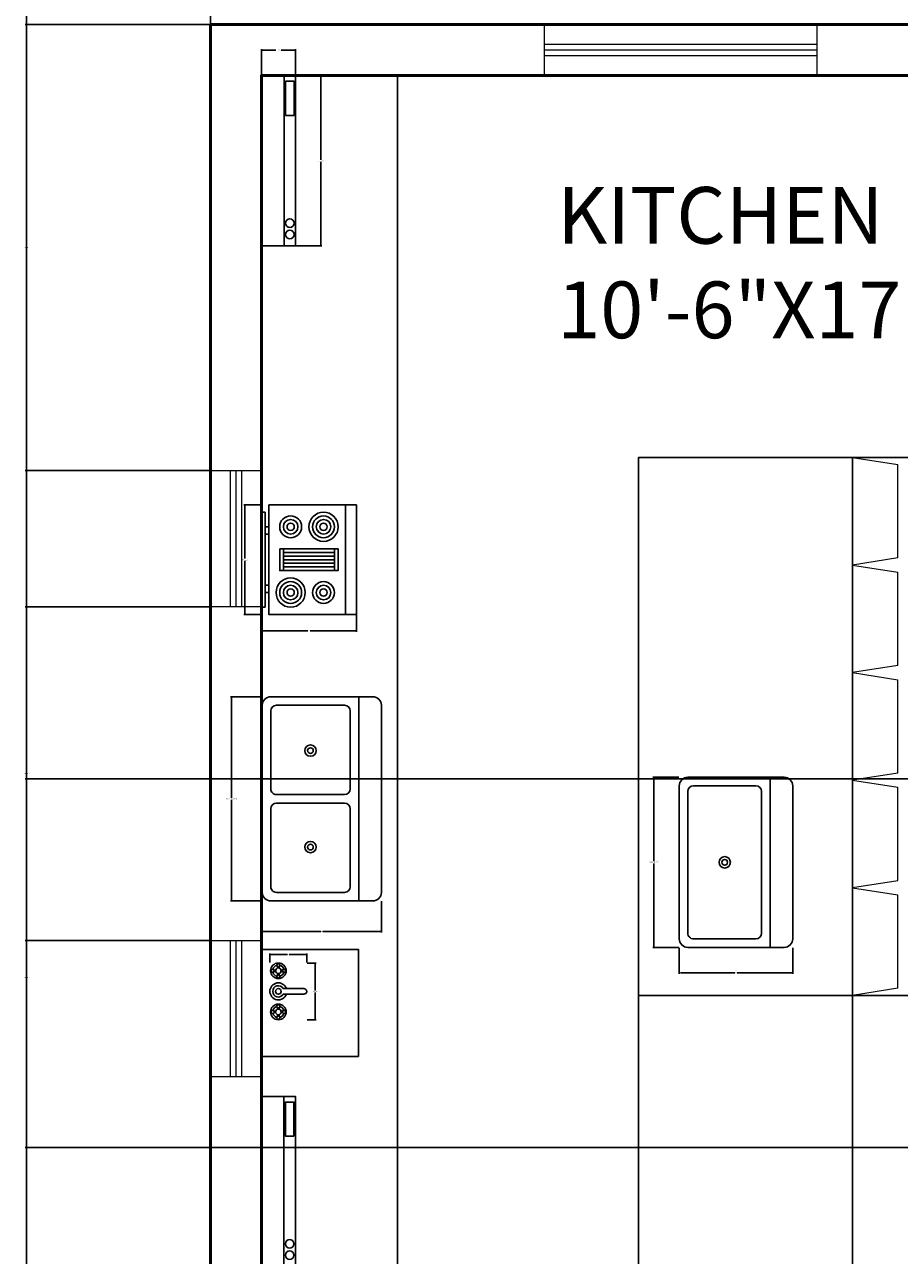
# Model space of a CAD drawing. Units: inches. Extents: x 821 to 2399, y 74 to 823.
# Tile 3 of 13: x 821 to 975, y 381 to 599. Entities that reach past the tile are written whole.
import ezdxf

# ---------------------------------------------------------------- set-up
doc = ezdxf.new("R2010")
doc.units = ezdxf.units.IN
doc.header["$MEASUREMENT"] = 0
doc.layers.get('0').update_dxf_attribs({"lineweight": 53})
for name, color, linetype, lineweight in [('A-ANNO-DIMS', 2, 'Continuous', 18), ('A-AREA-IDEN', 7, 'Continuous', 18), ('A-EQPM', 9, 'Continuous', 25), ('A-FLOR-CASE', 9, 'Continuous', 25), ('A-FLOR-FIXT', 8, 'Continuous', 25), ('A-FURN', 8, 'Continuous', 18), ('A-GLAZ', 4, 'Continuous', 18), ('WALLS', 7, 'Continuous', 50)]:
    doc.layers.add(name, color=color, linetype=linetype, lineweight=lineweight)
doc.styles.get("Standard").update_dxf_attribs({"font": 'arial.ttf'})
doc.dimstyles.get("Standard").update_dxf_attribs({"dimtxt": 0.18, "dimasz": 0.18, "dimexe": 0.18, "dimexo": 0.0625, "dimgap": 0.09, "dimtad": 0, "dimtih": 1, "dimtoh": 1, "dimdec": 4, "dimzin": 0, "dimdsep": 46, "dimtxsty": 'Standard', "dimcen": 0.09, "dimadec": 0, "dimazin": 0, "dimtfac": 1, "dimtdec": 4, "dimtofl": 0, "dimtmove": 0, "dimatfit": 3, "dimfxl": 1, "dimtolj": 1, "dimtzin": 0, "dimarcsym": 0})

# ---------------------------------------------------------------- blocks, each defined once
blk = doc.blocks.new('Faucet - Bathroom top')
for p, q in [((-4.107, 0.125), (-4.375, 0.125)), ((-3.75, 0.4788), (-3.75, 0.75)), ((-3.5, 0.482), (-3.5, 0.75)), ((-3.1461, 0.125), (-2.875, 0.125)), ((3.143, 0.125), (2.875, 0.125)), ((3.5, 0.4788), (3.5, 0.75)), ((3.75, 0.482), (3.75, 0.75)), ((4.1039, 0.125), (4.375, 0.125)), ((-4.1039, -0.125), (-4.375, -0.125)), ((-3.75, -0.4821), (-3.75, -0.75)), ((-3.5, -0.4789), (-3.5, -0.75)), ((-3.143, -0.125), (-2.875, -0.125)), ((-0.5, -0.8639), (-0.5, -4.5)), ((0.5, -4.5), (0.5, -0.8631)), ((3.1461, -0.125), (2.875, -0.125)), ((3.5, -0.4821), (3.5, -0.75)), ((3.75, -0.4789), (3.75, -0.75)), ((4.107, -0.125), (4.375, -0.125))]:
    blk.add_line(p, q)
for centre, radius in [((-3.625, 0), 1.375), ((-4.625, 0), 0.2795), ((-3.625, 0), 0.5), ((-3.625, 1), 0.2795), ((-2.625, 0), 0.2795), ((0, 0), 0.5), ((3.625, 0), 1.375), ((2.625, 0), 0.2795), ((3.625, 0), 0.5), ((3.625, 1), 0.2795), ((4.625, 0), 0.2795), ((-3.625, -1), 0.2795), ((3.625, -1), 0.2795)]:
    blk.add_circle(centre, radius)
for centre, radius, start, end in [((-3.625, 0), 1, 105.2407, 164.2093), ((-3.625, 0), 1, 16.44125, 74.07887), ((0, 0), 1.5, 289.6514, 250.3603), ((0, 0), 1, 300.3431, 239.7554), ((3.625, 0), 1, 106.12, 164.0884), ((3.625, 0), 1, 16.23422, 73.90469), ((-3.625, 0), 1, 196.2342, 253.9047), ((-3.625, 0), 1, 286.12, 344.0884), ((3.625, 0), 1, 196.4413, 254.0789), ((3.625, 0), 1, 285.2407, 344.2093), ((0, -4.5), 0.5, 180, 0)]:
    blk.add_arc(centre, radius, start, end)
blk = doc.blocks.new('Sink-single - 30 in top')
blk.add_line((-15, -3.999996), (15, -3.999996))
for points in [[(-13.5, 0), (13.5, 0)], [(-15, -18.499996), (-15, -1.5)], [(15, -1.5), (15, -18.499996)], [(-13.5, -17.499996), (-13.5, -6.499996)], [(-12.5, -5.499996), (12.5, -5.499996)], [(13.5, -6.499996), (13.5, -17.499996)], [(12.5, -18.499996), (-12.5, -18.499996)], [(13.5, -19.999996), (-13.5, -19.999996)]]:
    blk.add_lwpolyline(points)
for radius in [1, 0.5]:
    blk.add_circle((0, -11.999996), radius)
for centre, radius, start, end in [((-13.5, -1.5), 1.5, 90, 180), ((13.5, -1.5), 1.5, 0, 90), ((-12.5, -6.499996), 1, 90, 180), ((12.5, -6.499996), 1, 0, 90), ((-13.5, -18.499996), 1.5, 180, 270), ((-12.5, -17.499996), 1, 180, 270), ((12.5, -17.499996), 1, 270, 0), ((13.5, -18.499996), 1.5, 270, 0)]:
    blk.add_arc(centre, radius, start, end)
blk = doc.blocks.new('Sink-double - 36 in top')
for p, q in [((-18, -4), (18, -4)), ((-0.75, -18.5), (-0.75, -6.5)), ((0.75, -6.5), (0.75, -18.5))]:
    blk.add_line(p, q)
for points in [[(-16.5, 0), (16.5, 0)], [(-18, -19.5), (-18, -1.5)], [(18, -1.5), (18, -19.5)], [(-16.5, -18.5), (-16.5, -6.5)], [(-15.5, -5.5), (-1.75, -5.5)], [(1.75, -5.5), (15.5, -5.5)], [(16.5, -6.5), (16.5, -18.5)], [(-1.75, -19.5), (-15.5, -19.5)], [(15.5, -19.5), (1.75, -19.5)], [(16.5, -21), (-16.5, -21)]]:
    blk.add_lwpolyline(points)
for centre, radius in [((-8.5, -12.5), 1), ((-8.5, -12.5), 0.5), ((8.5, -12.5), 1), ((8.5, -12.5), 0.5)]:
    blk.add_circle(centre, radius)
for centre, radius, start, end in [((-16.5, -1.5), 1.5, 90, 180), ((16.5, -1.5), 1.5, 0, 90), ((-15.5, -6.5), 1, 90, 180), ((-1.75, -6.5), 1, 0, 90), ((1.75, -6.5), 1, 90, 180), ((15.5, -6.5), 1, 0, 90), ((-16.5, -19.5), 1.5, 180, 270), ((-15.5, -18.5), 1, 180, 270), ((-1.75, -18.5), 1, 270, 0), ((1.75, -18.5), 1, 180, 270), ((15.5, -18.5), 1, 270, 0), ((16.5, -19.5), 1.5, 270, 0)]:
    blk.add_arc(centre, radius, start, end)
blk = doc.blocks.new('Range-Oven - 30 in top')
for p, q in [((0, -3), (30, -3)), ((12, -6), (18, -6)), ((13, -20), (13, -6)), ((14, -6), (14, -20)), ((15, -20), (15, -6)), ((16, -6), (16, -20)), ((17, -20), (17, -6)), ((18, -20), (12, -20)), ((6, -24), (6, -25)), ((8, -25), (8, -24)), ((22, -25), (22, -24)), ((24, -24), (24, -25))]:
    blk.add_line(p, q)
for points in [[(0, -24), (0, 0), (30, 0), (30, -24)], [(12, -21), (12, -5), (18, -5), (18, -21)], [(2, -26), (2, -25), (28, -25), (28, -26)]]:
    blk.add_lwpolyline(points, close=True)
for centre, radius in [((6, -9), 4), ((6, -9), 3), ((24, -9), 3), ((6, -9), 2), ((6, -9), 1), ((24, -9), 2), ((24, -9), 1), ((6, -18), 3), ((6, -18), 2), ((24, -18), 4), ((24, -18), 3), ((24, -18), 2), ((6, -18), 1), ((24, -18), 1)]:
    blk.add_circle(centre, radius)
blk = doc.blocks.new('Range Hood - 30 in front')
blk.add_line((0, -4), (30.0001, -4))
for points in [[(0, -6), (0, 0), (30.0001, 0), (30.0001, -6)], [(23, -5.75), (23, -4.25), (29, -4.25), (29, -5.75)]]:
    blk.add_lwpolyline(points, close=True)
for centre in [(2, -5), (4, -5)]:
    blk.add_circle(centre, 0.75)
blk = doc.blocks.new('WIN-48IN')
for p, q in [((3.5, 48), (3.5, 0)), ((4.5, 48), (4.5, 0)), ((5.5, 48), (5.5, 0))]:
    blk.add_line(p, q)
blk.add_lwpolyline([(9, 0), (0, 0), (0, 48), (9, 48)], close=True)
blk = doc.blocks.new('WIN-24IN')
for p, q in [((3.5, 24), (3.5, 0)), ((4.5, 24), (4.5, 0)), ((5.5, 24), (5.5, 0))]:
    blk.add_line(p, q)
blk.add_lwpolyline([(0, 24), (9, 24), (9, 0), (0, 0)], close=True)
blk = doc.blocks.new('*D40')
at = {"layer": 'A-ANNO-DIMS', "color": 0, "lineweight": -2, "transparency": 16777216}
for p, q in [((868.44, 589.52), (873.05, 589.52)), ((872.87, 589.34), (872.87, 574.7)), ((872.87, 559.7), (872.87, 574.34)), ((868.44, 559.52), (873.05, 559.52))]:
    blk.add_line(p, q, dxfattribs=at)
at = {"layer": 'A-ANNO-DIMS', "color": 0, "lineweight": 50, "transparency": 16777216}
for points in [[(872.84, 589.34), (872.9, 589.34), (872.87, 589.52)], [(872.84, 559.7), (872.9, 559.7), (872.87, 559.52)]]:
    blk.add_solid(points, dxfattribs=at)
at = {"layer": 'Defpoints', "color": 0, "lineweight": 50, "transparency": 16777216}
for p in [(868.37, 589.52), (872.87, 589.52), (868.37, 559.52)]:
    blk.add_point(p, dxfattribs=at)
at = {"layer": 'A-ANNO-DIMS', "color": 0, "transparency": 16777216, "insert": (872.87, 574.52), "char_height": 0.18, "attachment_point": 5}
blk.add_mtext('\\A1;HOOD 30 TYP.', dxfattribs=at)
blk = doc.blocks.new('*D41')
at = {"layer": 'A-ANNO-DIMS', "color": 0, "lineweight": -2, "transparency": 16777216}
for p, q in [((862.37, 589.58), (862.37, 594.2)), ((862.55, 594.02), (864.91, 594.02)), ((868.19, 594.02), (865.83, 594.02)), ((868.37, 589.58), (868.37, 594.2))]:
    blk.add_line(p, q, dxfattribs=at)
at = {"layer": 'A-ANNO-DIMS', "color": 0, "lineweight": 50, "transparency": 16777216}
for points in [[(862.55, 594.05), (862.55, 593.99), (862.37, 594.02)], [(868.19, 594.05), (868.19, 593.99), (868.37, 594.02)]]:
    blk.add_solid(points, dxfattribs=at)
at = {"layer": 'Defpoints', "color": 0, "lineweight": 50, "transparency": 16777216}
for p in [(862.37, 594.02), (862.37, 589.52), (868.37, 589.52)]:
    blk.add_point(p, dxfattribs=at)
at = {"layer": 'A-ANNO-DIMS', "color": 0, "transparency": 16777216, "insert": (865.37, 594.02), "char_height": 0.18, "attachment_point": 5}
blk.add_mtext('\\A1;6 TYP.', dxfattribs=at)
blk = doc.blocks.new('*D58')
at = {"layer": 'A-ANNO-DIMS', "color": 0, "lineweight": -2, "transparency": 16777216}
for p, q in [((870.42, 433.03), (872.04, 433.03)), ((871.86, 432.85), (871.86, 428.21)), ((871.86, 423.21), (871.86, 427.85)), ((870.42, 423.03), (872.04, 423.03))]:
    blk.add_line(p, q, dxfattribs=at)
at = {"layer": 'A-ANNO-DIMS', "color": 0, "lineweight": 50, "transparency": 16777216}
for points in [[(871.83, 432.85), (871.89, 432.85), (871.86, 433.03)], [(871.83, 423.21), (871.89, 423.21), (871.86, 423.03)]]:
    blk.add_solid(points, dxfattribs=at)
at = {"layer": 'Defpoints', "color": 0, "lineweight": 50, "transparency": 16777216}
for p in [(870.36, 433.03), (871.86, 433.03), (870.36, 423.03)]:
    blk.add_point(p, dxfattribs=at)
at = {"layer": 'A-ANNO-DIMS', "color": 0, "transparency": 16777216, "insert": (871.86, 428.03), "char_height": 0.18, "attachment_point": 5}
blk.add_mtext('\\A1;TAP 10', dxfattribs=at)
blk = doc.blocks.new('*D59')
at = {"layer": 'A-ANNO-DIMS', "color": 0, "lineweight": -2, "transparency": 16777216}
for p, q in [((863.86, 433.1), (863.86, 434.71)), ((864.04, 434.53), (866.96, 434.53)), ((870.18, 434.53), (867.26, 434.53)), ((870.36, 433.1), (870.36, 434.71))]:
    blk.add_line(p, q, dxfattribs=at)
at = {"layer": 'A-ANNO-DIMS', "color": 0, "lineweight": 50, "transparency": 16777216}
for points in [[(864.04, 434.56), (864.04, 434.5), (863.86, 434.53)], [(870.18, 434.56), (870.18, 434.5), (870.36, 434.53)]]:
    blk.add_solid(points, dxfattribs=at)
at = {"layer": 'Defpoints', "color": 0, "lineweight": 50, "transparency": 16777216}
for p in [(863.86, 434.53), (863.86, 433.03), (870.36, 433.03)]:
    blk.add_point(p, dxfattribs=at)
at = {"layer": 'A-ANNO-DIMS', "color": 0, "transparency": 16777216, "insert": (867.11, 434.53), "char_height": 0.18, "attachment_point": 5}
blk.add_mtext('\\A1;7', dxfattribs=at)
blk = doc.blocks.new('*D60')
at = {"layer": 'A-ANNO-DIMS', "color": 0, "lineweight": -2, "transparency": 16777216}
for p, q in [((936, 465.79), (931.38, 465.79)), ((931.56, 465.61), (931.56, 450.97)), ((931.56, 435.97), (931.56, 450.6)), ((936, 435.79), (931.38, 435.79))]:
    blk.add_line(p, q, dxfattribs=at)
at = {"layer": 'A-ANNO-DIMS', "color": 0, "lineweight": 50, "transparency": 16777216}
for points in [[(931.53, 465.61), (931.59, 465.61), (931.56, 465.79)], [(931.53, 435.97), (931.59, 435.97), (931.56, 435.79)]]:
    blk.add_solid(points, dxfattribs=at)
at = {"layer": 'Defpoints', "color": 0, "lineweight": 50, "transparency": 16777216}
for p in [(936.06, 465.79), (931.56, 435.79), (936.06, 435.79)]:
    blk.add_point(p, dxfattribs=at)
at = {"layer": 'A-ANNO-DIMS', "color": 0, "transparency": 16777216, "insert": (931.56, 450.79), "char_height": 0.18, "attachment_point": 5}
blk.add_mtext('\\A1;ISLAND SINK 30', dxfattribs=at)
blk = doc.blocks.new('*D61')
at = {"layer": 'A-ANNO-DIMS', "color": 0, "lineweight": -2, "transparency": 16777216}
for p, q in [((936.06, 435.72), (936.06, 431.11)), ((956.06, 435.72), (956.06, 431.11)), ((936.24, 431.29), (945.84, 431.29)), ((955.88, 431.29), (946.28, 431.29))]:
    blk.add_line(p, q, dxfattribs=at)
at = {"layer": 'A-ANNO-DIMS', "color": 0, "lineweight": 50, "transparency": 16777216}
for points in [[(936.24, 431.32), (936.24, 431.26), (936.06, 431.29)], [(955.88, 431.32), (955.88, 431.26), (956.06, 431.29)]]:
    blk.add_solid(points, dxfattribs=at)
at = {"layer": 'Defpoints', "color": 0, "lineweight": 50, "transparency": 16777216}
for p in [(936.06, 435.79), (956.06, 435.79), (956.06, 431.29)]:
    blk.add_point(p, dxfattribs=at)
at = {"layer": 'A-ANNO-DIMS', "color": 0, "transparency": 16777216, "insert": (946.06, 431.29), "char_height": 0.18, "attachment_point": 5}
blk.add_mtext('\\A1;20', dxfattribs=at)
blk = doc.blocks.new('*D62')
at = {"layer": 'A-ANNO-DIMS', "color": 0, "lineweight": -2, "transparency": 16777216}
for p, q in [((862.46, 479.98), (856.94, 479.98)), ((857.12, 479.8), (857.12, 462.16)), ((857.12, 444.16), (857.12, 461.8)), ((862.46, 443.98), (856.94, 443.98))]:
    blk.add_line(p, q, dxfattribs=at)
at = {"layer": 'A-ANNO-DIMS', "color": 0, "lineweight": 50, "transparency": 16777216}
for points in [[(857.09, 479.8), (857.15, 479.8), (857.12, 479.98)], [(857.09, 444.16), (857.15, 444.16), (857.12, 443.98)]]:
    blk.add_solid(points, dxfattribs=at)
at = {"layer": 'Defpoints', "color": 0, "lineweight": 50, "transparency": 16777216}
for p in [(862.52, 479.98), (857.12, 443.98), (862.52, 443.98)]:
    blk.add_point(p, dxfattribs=at)
at = {"layer": 'A-ANNO-DIMS', "color": 0, "transparency": 16777216, "insert": (857.12, 461.98), "char_height": 0.18, "attachment_point": 5}
blk.add_mtext('\\A1;DOUBLE SINK 36', dxfattribs=at)
blk = doc.blocks.new('*D63')
at = {"layer": 'A-ANNO-DIMS', "color": 0, "lineweight": -2, "transparency": 16777216}
for p, q in [((862.52, 443.92), (862.52, 438.4)), ((883.52, 443.92), (883.52, 438.4)), ((862.7, 438.58), (872.82, 438.58)), ((883.34, 438.58), (873.22, 438.58))]:
    blk.add_line(p, q, dxfattribs=at)
at = {"layer": 'A-ANNO-DIMS', "color": 0, "lineweight": 50, "transparency": 16777216}
for points in [[(862.7, 438.61), (862.7, 438.55), (862.52, 438.58)], [(883.34, 438.61), (883.34, 438.55), (883.52, 438.58)]]:
    blk.add_solid(points, dxfattribs=at)
at = {"layer": 'Defpoints', "color": 0, "lineweight": 50, "transparency": 16777216}
for p in [(862.52, 443.98), (883.52, 443.98), (883.52, 438.58)]:
    blk.add_point(p, dxfattribs=at)
at = {"layer": 'A-ANNO-DIMS', "color": 0, "transparency": 16777216, "insert": (873.02, 438.58), "char_height": 0.18, "attachment_point": 5}
blk.add_mtext('\\A1;21', dxfattribs=at)
blk = doc.blocks.new('*D64')
at = {"layer": 'A-ANNO-DIMS', "color": 0, "lineweight": -2, "transparency": 16777216}
for p, q in [((862.31, 513.82), (859.29, 513.82)), ((859.47, 513.64), (859.47, 504.34)), ((859.47, 494.68), (859.47, 503.98)), ((862.31, 494.5), (859.29, 494.5))]:
    blk.add_line(p, q, dxfattribs=at)
at = {"layer": 'A-ANNO-DIMS', "color": 0, "lineweight": 50, "transparency": 16777216}
for points in [[(859.44, 513.64), (859.5, 513.64), (859.47, 513.82)], [(859.44, 494.68), (859.5, 494.68), (859.47, 494.5)]]:
    blk.add_solid(points, dxfattribs=at)
at = {"layer": 'Defpoints', "color": 0, "lineweight": 50, "transparency": 16777216}
for p in [(862.37, 513.82), (859.47, 494.5), (862.37, 494.5)]:
    blk.add_point(p, dxfattribs=at)
at = {"layer": 'A-ANNO-DIMS', "color": 0, "transparency": 16777216, "insert": (859.47, 504.16), "char_height": 0.18, "attachment_point": 5}
blk.add_mtext('\\A1;RANGE 19', dxfattribs=at)
blk = doc.blocks.new('*D65')
at = {"layer": 'A-ANNO-DIMS', "color": 0, "lineweight": -2, "transparency": 16777216}
for p, q in [((862.37, 494.44), (862.37, 491.42)), ((879.12, 494.44), (879.12, 491.42)), ((862.55, 491.6), (870.54, 491.6)), ((878.94, 491.6), (870.96, 491.6))]:
    blk.add_line(p, q, dxfattribs=at)
at = {"layer": 'A-ANNO-DIMS', "color": 0, "lineweight": 50, "transparency": 16777216}
for points in [[(862.55, 491.63), (862.55, 491.57), (862.37, 491.6)], [(878.94, 491.63), (878.94, 491.57), (879.12, 491.6)]]:
    blk.add_solid(points, dxfattribs=at)
at = {"layer": 'Defpoints', "color": 0, "lineweight": 50, "transparency": 16777216}
for p in [(862.37, 494.5), (879.12, 494.5), (879.12, 491.6)]:
    blk.add_point(p, dxfattribs=at)
at = {"layer": 'A-ANNO-DIMS', "color": 0, "transparency": 16777216, "insert": (870.75, 491.6), "char_height": 0.18, "attachment_point": 5}
blk.add_mtext('\\A1;17', dxfattribs=at)
blk = doc.blocks.new('*D80')
at = {"layer": 'A-ANNO-DIMS', "color": 0, "lineweight": -2, "transparency": 16777216}
for p, q in [((999.33, 754.12), (820.74, 754.12)), ((820.92, 753.94), (820.92, 430.67)), ((820.92, 107.04), (820.92, 430.31)), ((1050.58, 106.86), (820.74, 106.86))]:
    blk.add_line(p, q, dxfattribs=at)
at = {"layer": 'A-ANNO-DIMS', "color": 0, "lineweight": 50, "transparency": 16777216}
for points in [[(820.89, 753.94), (820.95, 753.94), (820.92, 754.12)], [(820.89, 107.04), (820.95, 107.04), (820.92, 106.86)]]:
    blk.add_solid(points, dxfattribs=at)
at = {"layer": 'Defpoints', "color": 0, "lineweight": 50, "transparency": 16777216}
for p in [(999.39, 754.12), (820.92, 106.86), (1050.64, 106.86)]:
    blk.add_point(p, dxfattribs=at)
at = {"layer": 'A-ANNO-DIMS', "color": 0, "transparency": 16777216, "insert": (820.92, 430.49), "char_height": 0.18, "attachment_point": 5}
blk.add_mtext('\\A1;647.3', dxfattribs=at)
blk = doc.blocks.new('*D81')
at = {"layer": 'A-ANNO-DIMS', "color": 0, "lineweight": -2, "transparency": 16777216}
for p, q in [((853.37, 292.61), (853.37, 786.75)), ((853.55, 786.57), (948.09, 786.57)), ((1043.19, 786.57), (948.65, 786.57)), ((1043.37, 292.58), (1043.37, 786.75))]:
    blk.add_line(p, q, dxfattribs=at)
at = {"layer": 'A-ANNO-DIMS', "color": 0, "lineweight": 50, "transparency": 16777216}
for points in [[(853.55, 786.6), (853.55, 786.54), (853.37, 786.57)], [(1043.19, 786.6), (1043.19, 786.54), (1043.37, 786.57)]]:
    blk.add_solid(points, dxfattribs=at)
at = {"layer": 'Defpoints', "color": 0, "lineweight": 50, "transparency": 16777216}
for p in [(1043.37, 786.57), (853.37, 292.55), (1043.37, 292.52)]:
    blk.add_point(p, dxfattribs=at)
at = {"layer": 'A-ANNO-DIMS', "color": 0, "transparency": 16777216, "insert": (948.37, 786.57), "char_height": 0.18, "attachment_point": 5}
blk.add_mtext('\\A1;190', dxfattribs=at)
blk = doc.blocks.new('*D97')
at = {"layer": 'A-ANNO-DIMS', "color": 0, "lineweight": -2, "transparency": 16777216}
for p, q in [((1152.31, 465.52), (820.74, 465.52)), ((820.92, 465.34), (820.92, 433.2)), ((820.92, 400.7), (820.92, 432.84)), ((1152.31, 400.52), (820.74, 400.52))]:
    blk.add_line(p, q, dxfattribs=at)
at = {"layer": 'A-ANNO-DIMS', "color": 0, "lineweight": 50, "transparency": 16777216}
for points in [[(820.89, 465.34), (820.95, 465.34), (820.92, 465.52)], [(820.89, 400.7), (820.95, 400.7), (820.92, 400.52)]]:
    blk.add_solid(points, dxfattribs=at)
at = {"layer": 'Defpoints', "color": 0, "lineweight": 50, "transparency": 16777216}
for p in [(820.92, 465.52), (1152.37, 465.52), (1152.37, 400.52)]:
    blk.add_point(p, dxfattribs=at)
at = {"layer": 'A-ANNO-DIMS', "color": 0, "transparency": 16777216, "insert": (820.92, 433.02), "char_height": 0.18, "attachment_point": 5}
blk.add_mtext('\\A1;65', dxfattribs=at)
blk = doc.blocks.new('*D101')
at = {"layer": 'A-ANNO-DIMS', "color": 0, "lineweight": -2, "transparency": 16777216}
for p, q in [((928.85, 427.27), (928.85, 74.23)), ((886.37, 379.46), (886.37, 74.23)), ((886.55, 74.41), (907.21, 74.41)), ((928.67, 74.41), (908.01, 74.41))]:
    blk.add_line(p, q, dxfattribs=at)
at = {"layer": 'A-ANNO-DIMS', "color": 0, "lineweight": 50, "transparency": 16777216}
for points in [[(886.55, 74.44), (886.55, 74.38), (886.37, 74.41)], [(928.67, 74.44), (928.67, 74.38), (928.85, 74.41)]]:
    blk.add_solid(points, dxfattribs=at)
at = {"layer": 'Defpoints', "color": 0, "lineweight": 50, "transparency": 16777216}
for p in [(928.85, 427.33), (886.37, 379.52), (928.85, 74.41)]:
    blk.add_point(p, dxfattribs=at)
at = {"layer": 'A-ANNO-DIMS', "color": 0, "transparency": 16777216, "insert": (907.61, 74.41), "char_height": 0.18, "attachment_point": 5}
blk.add_mtext('\\A1;42.48', dxfattribs=at)
blk = doc.blocks.new('*D102')
at = {"layer": 'A-ANNO-DIMS', "color": 0, "lineweight": -2, "transparency": 16777216}
for p, q in [((928.85, 427.27), (928.85, 74.23)), ((966.61, 427.27), (966.61, 74.23)), ((929.03, 74.41), (947.34, 74.41)), ((966.43, 74.41), (948.12, 74.41))]:
    blk.add_line(p, q, dxfattribs=at)
at = {"layer": 'A-ANNO-DIMS', "color": 0, "lineweight": 50, "transparency": 16777216}
for points in [[(929.03, 74.44), (929.03, 74.38), (928.85, 74.41)], [(966.43, 74.44), (966.43, 74.38), (966.61, 74.41)]]:
    blk.add_solid(points, dxfattribs=at)
at = {"layer": 'Defpoints', "color": 0, "lineweight": 50, "transparency": 16777216}
for p in [(928.85, 427.33), (966.61, 427.33), (966.61, 74.41)]:
    blk.add_point(p, dxfattribs=at)
at = {"layer": 'A-ANNO-DIMS', "color": 0, "transparency": 16777216, "insert": (947.73, 74.41), "char_height": 0.18, "attachment_point": 5}
blk.add_mtext('\\A1;37.76', dxfattribs=at)
blk = doc.blocks.new('*D103')
at = {"layer": 'A-ANNO-DIMS', "color": 0, "lineweight": -2, "transparency": 16777216}
for p, q in [((966.67, 522.18), (1330, 522.18)), ((1329.82, 522), (1329.82, 474.94)), ((1329.82, 427.51), (1329.82, 474.57)), ((966.67, 427.33), (1330, 427.33))]:
    blk.add_line(p, q, dxfattribs=at)
at = {"layer": 'A-ANNO-DIMS', "color": 0, "lineweight": 50, "transparency": 16777216}
for points in [[(1329.79, 522), (1329.85, 522), (1329.82, 522.18)], [(1329.79, 427.51), (1329.85, 427.51), (1329.82, 427.33)]]:
    blk.add_solid(points, dxfattribs=at)
at = {"layer": 'Defpoints', "color": 0, "lineweight": 50, "transparency": 16777216}
for p in [(966.61, 522.18), (1329.82, 522.18), (966.61, 427.33)]:
    blk.add_point(p, dxfattribs=at)
at = {"layer": 'A-ANNO-DIMS', "color": 0, "transparency": 16777216, "insert": (1329.82, 474.75), "char_height": 0.18, "attachment_point": 5}
blk.add_mtext('\\A1;94.85', dxfattribs=at)
blk = doc.blocks.new('*D105')
at = {"layer": 'A-ANNO-DIMS', "color": 0, "lineweight": -2, "transparency": 16777216}
for p, q in [((853.31, 598.52), (820.74, 598.52)), ((820.92, 598.34), (820.92, 559.38)), ((820.92, 520.05), (820.92, 559.01)), ((853.31, 519.87), (820.74, 519.87))]:
    blk.add_line(p, q, dxfattribs=at)
at = {"layer": 'A-ANNO-DIMS', "color": 0, "lineweight": 50, "transparency": 16777216}
for points in [[(820.89, 598.34), (820.95, 598.34), (820.92, 598.52)], [(820.89, 520.05), (820.95, 520.05), (820.92, 519.87)]]:
    blk.add_solid(points, dxfattribs=at)
at = {"layer": 'Defpoints', "color": 0, "lineweight": 50, "transparency": 16777216}
for p in [(853.37, 598.52), (820.92, 519.87), (853.37, 519.87)]:
    blk.add_point(p, dxfattribs=at)
at = {"layer": 'A-ANNO-DIMS', "color": 0, "transparency": 16777216, "insert": (820.92, 559.2), "char_height": 0.18, "attachment_point": 5}
blk.add_mtext('\\A1;78.65', dxfattribs=at)
blk = doc.blocks.new('*D106')
at = {"layer": 'A-ANNO-DIMS', "color": 0, "lineweight": -2, "transparency": 16777216}
for p, q in [((853.31, 495.87), (820.74, 495.87)), ((820.92, 495.69), (820.92, 466.61)), ((820.92, 437.16), (820.92, 466.25)), ((853.31, 436.98), (820.74, 436.98))]:
    blk.add_line(p, q, dxfattribs=at)
at = {"layer": 'A-ANNO-DIMS', "color": 0, "lineweight": 50, "transparency": 16777216}
for points in [[(820.89, 495.69), (820.95, 495.69), (820.92, 495.87)], [(820.89, 437.16), (820.95, 437.16), (820.92, 436.98)]]:
    blk.add_solid(points, dxfattribs=at)
at = {"layer": 'Defpoints', "color": 0, "lineweight": 50, "transparency": 16777216}
for p in [(853.37, 495.87), (820.92, 436.98), (853.37, 436.98)]:
    blk.add_point(p, dxfattribs=at)
at = {"layer": 'A-ANNO-DIMS', "color": 0, "transparency": 16777216, "insert": (820.92, 466.43), "char_height": 0.18, "attachment_point": 5}
blk.add_mtext('\\A1;58.89', dxfattribs=at)

msp = doc.modelspace()

# ---------------------------------------------------------------- linework, layer by layer
at = {"layer": 'A-FLOR-CASE'}
msp.add_line((886.3735, 589.5195), (886.3735, 379.5195), dxfattribs=at)
msp.add_lwpolyline([(966.6107, 517.0239), (966.6107, 427.3294), (928.8511, 427.3294), (928.8511, 517.0239), (928.8511, 522.1769), (966.6107, 522.1769)], close=True, dxfattribs=at)
at = {"layer": 'A-FLOR-FIXT'}
msp.add_lwpolyline([(862.3735, 435.4419), (879.483, 435.4419), (879.483, 416.5646), (862.3735, 416.5646)], close=True, dxfattribs=at)
at = {"layer": 'A-FURN'}
for p, q in [((966.6107, 522.1769), (974.6124, 520.9266)), ((974.6131, 504.4617), (974.6131, 520.9313)), ((974.6131, 485.4922), (974.6131, 501.9618)), ((974.6131, 466.5227), (974.6131, 482.9923)), ((974.6131, 447.5532), (974.6131, 464.0228)), ((974.6131, 428.5837), (974.6131, 445.0533)), ((974.6137, 428.5798), (966.6107, 427.3294))]:
    msp.add_line(p, q, dxfattribs=at)
for points in [[(974.6137, 504.4578), (966.6107, 503.2074), (974.6124, 501.9571)], [(974.6137, 485.4883), (966.6107, 484.2379), (974.6124, 482.9876)], [(974.6137, 466.5188), (966.6107, 465.2684), (974.6124, 464.0181)], [(974.6137, 447.5493), (966.6107, 446.2989), (974.6124, 445.0486)]]:
    msp.add_lwpolyline(points, dxfattribs=at)
at = {"layer": 'WALLS'}
msp.add_lwpolyline([(1050.641, 200.5195), (1050.641, 170.9407), (1121.9086, 170.9407), (1128.124, 170.9407), (1050.641, 170.9407), (1050.641, 106.8645), (1128.124, 106.8645), (1128.124, 170.9407), (1128.124, 200.5195), (1288.3735, 200.5195), (1297.3735, 200.5195), (1297.3735, 598.5195), (853.3735, 598.5195), (853.3735, 292.549), (922.3673, 292.5195), (1043.3735, 292.5195), (1043.3735, 209.5195), (1043.3735, 200.5195)], close=True, dxfattribs=at)
for points in [[(862.3735, 379.5195), (862.3735, 589.5195), (862.3735, 379.5195), (888.3735, 379.5195)], [(862.3735, 589.5195), (1148.3735, 589.5195), (1148.3735, 563.3933), (1148.3735, 565.3933), (1150.3735, 565.3933), (1150.3735, 563.3933), (1174.3735, 563.3933)]]:
    msp.add_lwpolyline(points, dxfattribs=at)

# ---------------------------------------------------------------- block references
at = {"layer": 'A-EQPM', "rotation": 90}
for p in [(862.3735, 559.5194), (862.3528, 379.5195)]:
    msp.add_blockref('Range Hood - 30 in front', p, dxfattribs=at)
at = {"layer": 'A-EQPM', "xscale": 0.6442159420823373, "yscale": 0.6442159420823373, "zscale": 0.6442159420823373, "rotation": 270}
msp.add_blockref('Range-Oven - 30 in top', (879.1231, 513.8249), dxfattribs=at)
at = {"layer": 'A-FLOR-FIXT'}
for name, p, rotation in [('Sink-double - 36 in top', (883.5205, 461.9804), 270), ('Sink-single - 30 in top', (956.0586, 450.7864), 270), ('Faucet - Bathroom top', (865.3603, 428.0326), 90)]:
    msp.add_blockref(name, p, dxfattribs=dict(at, rotation=rotation))
at = {"layer": 'A-GLAZ', "rotation": 269.9999999999984}
msp.add_blockref('WIN-48IN', (912.3016, 598.5199), dxfattribs=at)
at = {"layer": 'A-GLAZ'}
for p in [(853.373, 495.873), (853.373, 412.9839)]:
    msp.add_blockref('WIN-24IN', p, dxfattribs=at)

# ---------------------------------------------------------------- texts
at = {"layer": 'A-AREA-IDEN', "insert": (914.5519, 569.8843), "char_height": 10, "attachment_point": 1}
msp.add_mtext_dynamic_manual_height_columns('KITCHEN\\P10\'-6"X17\'-10"', width=75.475047, gutter_width=1, heights=[0], dxfattribs=at)

# ---------------------------------------------------------------- dimensions: what is measured, and where the dimension line sits
at = {"layer": 'A-ANNO-DIMS'}
for base, p1, p2, override, picture, middle in [((1043.3735, 786.5664), (853.3735, 292.549), (1043.3735, 292.5195), {"dimdec": 0, "dimlfac": 1, "dimrnd": 0, "dimzin": 0, "dimdsep": 46, "dimlunit": 2}, '*D81', (948.3735, 786.5664)), ((879.1231, 491.5994), (862.3735, 494.4984), (879.1231, 494.4984), {"dimdec": 0, "dimlfac": 1, "dimrnd": 0, "dimzin": 0, "dimdsep": 46, "dimlunit": 2}, '*D65', (870.7483, 491.5994)), ((883.5205, 438.5804), (862.5205, 443.9804), (883.5205, 443.9804), {"dimdec": 0, "dimlfac": 1, "dimrnd": 0, "dimzin": 0, "dimdsep": 46, "dimlunit": 2}, '*D63', (873.0205, 438.5804)), ((956.0586, 431.2864), (936.0586, 435.7864), (956.0586, 435.7864), {"dimdec": 0, "dimlfac": 1, "dimrnd": 0, "dimzin": 0, "dimdsep": 46, "dimlunit": 2}, '*D61', (946.0586, 431.2864)), ((928.8511, 74.4145), (886.3735, 379.5195), (928.8511, 427.3294), {"dimdec": 2, "dimlfac": 1, "dimrnd": 0, "dimzin": 0, "dimdsep": 46, "dimlunit": 2}, '*D101', (907.6123, 74.4145)), ((966.6107, 74.4145), (928.8511, 427.3294), (966.6107, 427.3294), {"dimdec": 2, "dimlfac": 1, "dimrnd": 0, "dimzin": 0, "dimdsep": 46, "dimlunit": 2}, '*D102', (947.7309, 74.4145))]:
    dim = msp.add_linear_dim(base=base, p1=p1, p2=p2, dimstyle='Standard', override=override, dxfattribs=at)
    dim.commit()
    dim.dimension.update_dxf_attribs({"geometry": picture, "text_midpoint": middle})
for base, p1, p2, angle, override, picture, middle in [((820.9235, 106.8645), (999.3938, 754.1164), (1050.641, 106.8645), 90, {"dimdec": 1, "dimlfac": 1, "dimrnd": 0, "dimzin": 0, "dimdsep": 46, "dimlunit": 2}, '*D80', (820.9235, 430.4905)), ((820.9235, 519.8734), (853.3735, 598.5195), (853.3735, 519.8734), 90, {"dimdec": 2, "dimlfac": 1, "dimrnd": 0, "dimzin": 0, "dimdsep": 46, "dimlunit": 2}, '*D105', (820.9235, 559.1964)), ((1329.8235, 522.1769), (966.6107, 427.3294), (966.6107, 522.1769), 90, {"dimdec": 2, "dimlfac": 1, "dimrnd": 0, "dimzin": 0, "dimdsep": 46, "dimlunit": 2}, '*D103', (1329.8235, 474.7531)), ((820.9235, 436.9842), (853.3735, 495.8734), (853.3735, 436.9842), 90, {"dimdec": 2, "dimlfac": 1, "dimrnd": 0, "dimzin": 0, "dimdsep": 46, "dimlunit": 2}, '*D106', (820.9235, 466.4288)), ((820.9235, 465.5195), (1152.3735, 400.5195), (1152.3735, 465.5195), 90, {"dimdec": 0, "dimlfac": 1, "dimrnd": 0, "dimzin": 0, "dimdsep": 46, "dimlunit": 2}, '*D97', (820.9235, 433.0195)), ((863.8602, 434.5326), (870.3603, 433.0326), (863.8602, 433.0326), 180, {"dimdec": 0, "dimlfac": 1, "dimrnd": 0, "dimzin": 0, "dimdsep": 46, "dimlunit": 2}, '*D59', (867.1103, 434.5326))]:
    dim = msp.add_linear_dim(base=base, p1=p1, p2=p2, angle=angle, dimstyle='Standard', override=override, dxfattribs=at)
    dim.commit()
    dim.dimension.update_dxf_attribs({"geometry": picture, "text_midpoint": middle})
for base, p1, p2, angle, text, picture, middle in [((862.3735, 594.0195), (868.3735, 589.5195), (862.3735, 589.5195), 180, '<> TYP.', '*D41', (865.3735, 594.0195)), ((872.8735, 589.5195), (868.3735, 559.5194), (868.3735, 589.5195), 90, 'HOOD <> TYP.', '*D40', (872.8735, 574.5194)), ((859.4745, 494.4984), (862.3735, 513.8249), (862.3735, 494.4984), 270, 'RANGE <>', '*D64', (859.4745, 504.1616)), ((857.1205, 443.9804), (862.5205, 479.9804), (862.5205, 443.9804), 270, 'DOUBLE SINK <>', '*D62', (857.1205, 461.9804)), ((931.5586, 435.7864), (936.0586, 465.7864), (936.0586, 435.7864), 270, 'ISLAND SINK <>', '*D60', (931.5586, 450.7864)), ((871.8603, 433.0326), (870.3603, 423.0326), (870.3603, 433.0326), 90, 'TAP <>', '*D58', (871.8603, 428.0326))]:
    dim = msp.add_linear_dim(base=base, p1=p1, p2=p2, angle=angle, text=text, dimstyle='Standard', override={"dimdec": 0, "dimlfac": 1, "dimrnd": 0, "dimzin": 0, "dimdsep": 46, "dimlunit": 2}, dxfattribs=at)
    dim.commit()
    dim.dimension.update_dxf_attribs({"geometry": picture, "text_midpoint": middle})

doc.saveas('drawing.dxf')
